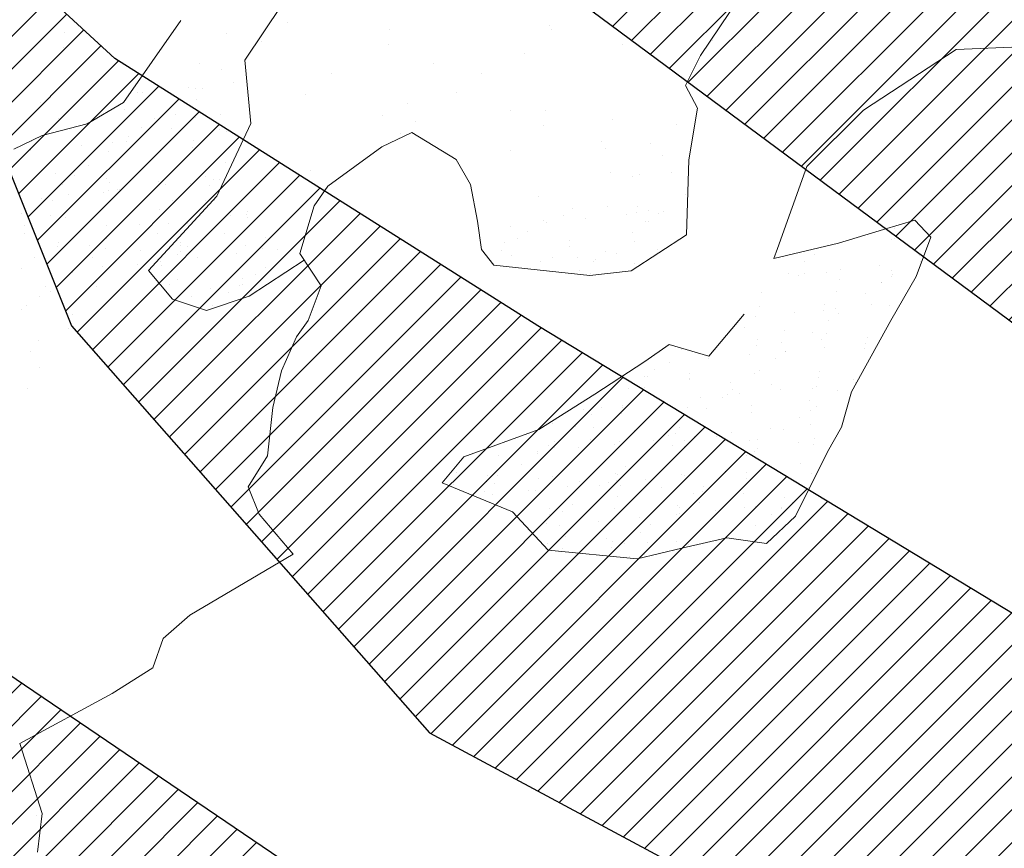
# Model space of a CAD drawing. Units: inches. Extents: x 1986 to 21484, y -1816 to 2016.
# Tile 63 of 85: x 3655.81 to 3662.33, y 1889.501 to 1894.988. Entities that reach past the tile are written whole.
import ezdxf

# ---------------------------------------------------------------- set-up
doc = ezdxf.new("R2010")
doc.units = ezdxf.units.IN
doc.layers.add('L-PLNT', color=84, linetype='Continuous', lineweight=13)
doc.layers.add('vfolhas', color=114, linetype='Continuous', lineweight=5)
doc.layers.add('vfolha2', color=110, linetype='Continuous')
doc.layers.add('vfolhas2', color=102, linetype='Continuous')
pattern_1 = [(45, (-2446.5133113, 50.986076), (-0.004419417382, 0.004419417382), [])]

# ---------------------------------------------------------------- blocks, each defined once
blk = doc.blocks.new('arbusto_PB_verde_grande')
at = {"layer": 'vfolha2'}
h = blk.add_hatch(dxfattribs=at)
h.set_pattern_fill('ANSI31', color=256, scale=0.05, style=0)
h.set_pattern_definition(pattern_1)
h.paths.add_polyline_path([(0.02944, 0.35651), (0.00028, 0.09048), (0.02625, -0.03934), (0.047, 0.06233), (0.06189, 0.09731), (0.09372, 0.26573), (0.09955, 0.43473), (0.08789, 0.61313), (0.0645, 0.72266), (0.04988, 0.6851), (0.0236, 0.51294)])
h.paths.add_polyline_path([(0.30106, 0.43789), (0.14225, 0.24871), (0.26685, 0.30022)])
h.paths.add_polyline_path([(0.37995, 0.22817), (0.23697, 0.15193), (0.18428, 0.09364), (0.11122, 0.04358), (0.02625, -0.03934), (0.28061, 0.04667), (0.36829, 0.07798), (0.46756, 0.11239), (0.61068, 0.19376), (0.71585, 0.27823), (0.55813, 0.25948)])
h.paths.add_polyline_path([(0.56101, -0.29441), (0.72752, -0.32573), (0.59024, -0.2412), (0.42962, -0.15982), (0.02625, -0.03934), (0.14922, -0.14107), (0.18838, -0.16604), (0.41501, -0.24435)])
h.paths.add_polyline_path([(-0.27429, -0.44776), (-0.30352, -0.72628), (-0.23923, -0.64175), (-0.15457, -0.45716), (0.02625, -0.03934), (-0.16328, -0.25376)])
h.paths.add_polyline_path([(-0.51963, -0.24744), (-0.67736, -0.32573), (-0.59558, -0.35072), (-0.40574, -0.32882), (-0.21007, -0.20995), (0.02625, -0.03934), (-0.14874, -0.06595), (-0.31518, -0.09101), (-0.41452, -0.15048)])
h.paths.add_polyline_path([(-0.52546, 0.25007), (-0.70947, 0.24698), (-0.51963, 0.1093), (-0.32979, 0.02167), (-0.07567, -0.0128), (-0.04234, -0.02148), (-0.35024, 0.1312)])
h = blk.add_hatch(dxfattribs=at)
h.set_pattern_fill('ANSI31', color=256, scale=0.05, style=0)
h.set_pattern_definition(pattern_1)
h.paths.add_polyline_path([(-0.18963, 0.29704), (-0.08553, 0.20192), (-0.10785, 0.25007), (-0.13202, 0.31865), (-0.25096, 0.48479), (-0.44952, 0.5505), (-0.37946, 0.43789)])
h.paths.add_polyline_path([(0.07911, -0.4071), (0.08214, -0.50631), (0.17255, -0.6355), (0.18428, -0.44151), (0.14904, -0.29177), (0.02625, -0.03934), (0.03527, -0.25376)])
at = {"layer": 'vfolhas'}
h = blk.add_hatch(dxfattribs=at)
h.set_pattern_fill('ANSI31', color=256, scale=0.05, style=0)
h.set_pattern_definition(pattern_1)
h.paths.add_polyline_path([(-0.07279, 0.50669), (-0.18085, 0.65063), (-0.2334, 0.67253), (-0.20712, 0.53176), (-0.10785, 0.25007), (0.02625, -0.03934), (0.00028, 0.09048), (0.00816, 0.16241), (-0.04939, 0.29079)])
h.paths.add_polyline_path([(0.09902, 0.41929), (0.09372, 0.26573), (0.07906, 0.18814), (0.15506, 0.36901), (0.26606, 0.5505), (0.28356, 0.63504), (0.2485, 0.68819), (0.25145, 0.63504), (0.20178, 0.54426)])
h.paths.add_polyline_path([(0.12295, 0.24073), (0.047, 0.06233), (0.02625, -0.03934), (0.11122, 0.04358), (0.18428, 0.09364), (0.27478, 0.19376), (0.3215, 0.25323), (0.44129, 0.38467), (0.47634, 0.57866), (0.41789, 0.45347), (0.28939, 0.30954)])
h.paths.add_polyline_path([(0.58145, -0.03779), (0.70707, 0.01536), (0.78591, 0.04667), (0.74796, 0.06549), (0.62818, 0.08423), (0.52595, 0.09048), (0.39745, 0.04358), (0.02625, -0.03934), (0.25728, -0.03154), (0.43834, -0.0347)])
h.paths.add_polyline_path([(0.52022, -0.03647), (0.43834, -0.0347), (0.25728, -0.03154), (0.02625, -0.03934), (0.17964, -0.08515), (0.53768, -0.13167), (0.69541, -0.15357), (0.78591, -0.07852), (0.70413, -0.10042)])
h.paths.add_polyline_path([(0.27189, -0.21929), (0.14922, -0.14107), (0.02625, -0.03934), (0.15794, -0.31007), (0.29522, -0.42585), (0.41789, -0.49157), (0.56396, -0.56669), (0.5114, -0.48532), (0.39456, -0.34139)])
h.paths.add_polyline_path([(-0.05818, -0.47591), (-0.02312, -0.61984), (0.047, -0.80134), (0.08494, -0.59794), (0.07911, -0.4071), (0.03527, -0.25376), (0.02625, -0.03934), (-0.03773, -0.26001)])
h.paths.add_polyline_path([(-0.24218, 0.14054), (-0.11073, 0.06858), (0.02625, -0.03934), (-0.04235, 0.10871), (-0.21007, 0.23757), (-0.36485, 0.33145), (-0.47874, 0.40341), (-0.54303, 0.46288), (-0.49041, 0.33145), (-0.39408, 0.22192)])
at = {"layer": 'vfolha2'}
for p, q in [((-0.37946, 0.43789), (-0.18963, 0.29704)), ((-0.52546, 0.25007), (-0.35024, 0.1312))]:
    blk.add_line(p, q, dxfattribs=at)
at = {"layer": 'vfolhas2'}
for p, q in [((-0.54303, 0.46288), (-0.49041, 0.33145)), ((-0.47874, 0.40341), (-0.54303, 0.46288)), ((-0.36485, 0.33145), (-0.47874, 0.40341)), ((-0.49041, 0.33145), (-0.39408, 0.22192)), ((-0.21007, 0.23757), (-0.36485, 0.33145)), ((-0.39408, 0.22192), (-0.24218, 0.14054))]:
    blk.add_line(p, q, dxfattribs=at)
blk = doc.blocks.new('PLANT-SHRUB')
for p, q in [((2164.0917, 1878.6487), (2164.5363, 1878.8153)), ((2164.5363, 1878.8153), (2164.8003, 1878.8153)), ((2164.8003, 1878.8153), (2164.967, 1878.607)), ((2164.8003, 1878.8153), (2164.8003, 1878.8153)), ((2164.3454, 1878.7354), (2164.3454, 1878.7354)), ((2164.4894, 1878.7345), (2164.4894, 1878.7345)), ((2164.2631, 1878.6802), (2164.2631, 1878.6802)), ((2164.5043, 1878.672), (2164.5043, 1878.672)), ((2164.5625, 1878.7068), (2164.5625, 1878.7068)), ((2164.5717, 1878.7149), (2164.5717, 1878.7149)), ((2164.6457, 1878.6958), (2164.6457, 1878.6958)), ((2164.7757, 1878.6787), (2164.7757, 1878.6787)), ((2164.9028, 1878.6857), (2164.9028, 1878.6857)), ((2163.9111, 1878.5931), (2164.0917, 1878.6487)), ((2164.967, 1878.607), (2165.231, 1878.4543)), ((2163.7026, 1878.4682), (2163.9111, 1878.5931)), ((2164.124, 1878.5527), (2164.124, 1878.5527)), ((2164.2732, 1878.5846), (2164.2732, 1878.5846)), ((2164.6821, 1878.5866), (2164.6821, 1878.5866)), ((2164.7437, 1878.5398), (2164.7437, 1878.5398)), ((2163.1885, 1878.3016), (2163.7026, 1878.4682)), ((2163.7026, 1878.4682), (2163.7026, 1878.4682)), ((2164.0946, 1878.5257), (2164.0946, 1878.5257)), ((2164.1874, 1878.4701), (2164.1874, 1878.4701)), ((2164.6853, 1878.4692), (2164.6853, 1878.4692)), ((2165.1831, 1878.4683), (2165.1831, 1878.4683)), ((2163.6377, 1878.4146), (2163.6377, 1878.4146)), ((2163.6385, 1878.4401), (2163.6385, 1878.4401)), ((2164.0475, 1878.4421), (2164.0475, 1878.4421)), ((2164.4793, 1878.4265), (2164.4793, 1878.4265)), ((2164.6046, 1878.4124), (2164.6046, 1878.4124)), ((2164.8978, 1878.4212), (2164.8978, 1878.4212)), ((2165.2243, 1878.3995), (2165.2243, 1878.3995)), ((2165.231, 1878.4543), (2165.495, 1878.3016)), ((2163.7676, 1878.3975), (2163.7676, 1878.3975)), ((2163.9355, 1878.3799), (2163.9355, 1878.3799)), ((2163.9848, 1878.3689), (2163.9848, 1878.3689)), ((2164.068, 1878.358), (2164.068, 1878.358)), ((2164.198, 1878.3409), (2164.198, 1878.3409)), ((2164.5752, 1878.3854), (2164.5752, 1878.3854)), ((2162.869, 1878.2044), (2163.1885, 1878.3016)), ((2163.1885, 1878.3016), (2163.1885, 1878.3016)), ((2163.3794, 1878.2735), (2163.3794, 1878.2735)), ((2163.4129, 1878.2975), (2163.4129, 1878.2975)), ((2163.4468, 1878.3164), (2163.4468, 1878.3164)), ((2163.8446, 1878.2819), (2163.8446, 1878.2819)), ((2163.8773, 1878.2725), (2163.8773, 1878.2725)), ((2163.9447, 1878.3155), (2163.9447, 1878.3155)), ((2164.2631, 1878.2766), (2164.2631, 1878.2766)), ((2164.3751, 1878.2716), (2164.3751, 1878.2716)), ((2164.4151, 1878.3123), (2164.4151, 1878.3123)), ((2164.4426, 1878.3146), (2164.4426, 1878.3146)), ((2164.4983, 1878.3013), (2164.4983, 1878.3013)), ((2164.6283, 1878.2842), (2164.6283, 1878.2842)), ((2164.6721, 1878.2786), (2164.6721, 1878.2786)), ((2164.873, 1878.2707), (2164.873, 1878.2707)), ((2164.9404, 1878.3137), (2164.9404, 1878.3137)), ((2165.0852, 1878.2721), (2165.0852, 1878.2721)), ((2165.3708, 1878.2698), (2165.3708, 1878.2698)), ((2165.4383, 1878.3128), (2165.4383, 1878.3128)), ((2165.495, 1878.3016), (2165.8841, 1877.8573)), ((2162.6189, 1878.0794), (2162.869, 1878.2044)), ((2163.1272, 1878.22), (2163.1272, 1878.22)), ((2163.1272, 1878.22), (2163.1272, 1878.22)), ((2163.7669, 1878.2255), (2163.7669, 1878.2255)), ((2163.7964, 1878.2525), (2163.7964, 1878.2525)), ((2164.416, 1878.2396), (2164.416, 1878.2396)), ((2164.8455, 1878.2556), (2164.8455, 1878.2556)), ((2164.9287, 1878.2447), (2164.9287, 1878.2447)), ((2165.0558, 1878.2451), (2165.0558, 1878.2451)), ((2165.0586, 1878.2275), (2165.0586, 1878.2275)), ((2165.1039, 1878.263), (2165.1039, 1878.263)), ((2165.5223, 1878.2577), (2165.5223, 1878.2577)), ((2162.7782, 1878.153), (2162.7782, 1878.153)), ((2165.2758, 1878.199), (2165.2758, 1878.199)), ((2165.359, 1878.188), (2165.359, 1878.188)), ((2165.489, 1878.1709), (2165.489, 1878.1709)), ((2162.6189, 1877.9267), (2162.6189, 1878.0794)), ((2162.7596, 1878.1163), (2162.7596, 1878.1163)), ((2162.9767, 1878.0877), (2162.9767, 1878.0877)), ((2162.9767, 1878.0877), (2162.9767, 1878.0877)), ((2162.9881, 1878.0925), (2162.9881, 1878.0925)), ((2162.9881, 1878.0925), (2162.9881, 1878.0925)), ((2163.0599, 1878.0768), (2163.0599, 1878.0768)), ((2163.0599, 1878.0768), (2163.0599, 1878.0768)), ((2163.21, 1878.1374), (2163.21, 1878.1374)), ((2163.6078, 1878.0796), (2163.6078, 1878.0796)), ((2163.6285, 1878.1321), (2163.6285, 1878.1321)), ((2164.0374, 1878.134), (2164.0374, 1878.134)), ((2164.2475, 1878.0851), (2164.2475, 1878.0851)), ((2164.277, 1878.1121), (2164.277, 1878.1121)), ((2164.4692, 1878.1185), (2164.4692, 1878.1185)), ((2164.8877, 1878.1131), (2164.8877, 1878.1131)), ((2164.8966, 1878.0993), (2164.8966, 1878.0993)), ((2165.2966, 1878.1151), (2165.2966, 1878.1151)), ((2165.5363, 1878.1048), (2165.5363, 1878.1048)), ((2165.5658, 1878.1318), (2165.5658, 1878.1318)), ((2162.9587, 1878.0655), (2162.9587, 1878.0655)), ((2162.9587, 1878.0655), (2162.9587, 1878.0655)), ((2163.0626, 1878.0716), (2163.0626, 1878.0716)), ((2163.0626, 1878.0716), (2163.0626, 1878.0716)), ((2163.1899, 1878.0596), (2163.1899, 1878.0596)), ((2163.4071, 1878.0311), (2163.4071, 1878.0311)), ((2163.4903, 1878.0201), (2163.4903, 1878.0201)), ((2163.5604, 1878.0707), (2163.5604, 1878.0707)), ((2164.0583, 1878.0698), (2164.0583, 1878.0698)), ((2164.5561, 1878.0689), (2164.5561, 1878.0689)), ((2165.054, 1878.068), (2165.054, 1878.068)), ((2165.5518, 1878.0671), (2165.5518, 1878.0671)), ((2162.9938, 1877.9875), (2162.9938, 1877.9875)), ((2162.9938, 1877.9875), (2162.9938, 1877.9875)), ((2163.4028, 1877.9895), (2163.4028, 1877.9895)), ((2163.4687, 1877.9522), (2163.4687, 1877.9522)), ((2163.6202, 1878.003), (2163.6202, 1878.003)), ((2163.8346, 1877.9739), (2163.8346, 1877.9739)), ((2163.8374, 1877.9744), (2163.8374, 1877.9744)), ((2163.9206, 1877.9634), (2163.9206, 1877.9634)), ((2164.0506, 1877.9463), (2164.0506, 1877.9463)), ((2164.253, 1877.9686), (2164.253, 1877.9686)), ((2164.662, 1877.9705), (2164.662, 1877.9705)), ((2164.7281, 1877.9448), (2164.7281, 1877.9448)), ((2164.7575, 1877.9718), (2164.7575, 1877.9718)), ((2165.0938, 1877.955), (2165.0938, 1877.955)), ((2165.3772, 1877.959), (2165.3772, 1877.959)), ((2165.5123, 1877.9496), (2165.5123, 1877.9496)), ((2162.8134, 1877.8295), (2162.6189, 1877.9267)), ((2162.7995, 1877.9197), (2162.7995, 1877.9197)), ((2162.7995, 1877.9197), (2162.7995, 1877.9197)), ((2162.8199, 1877.917), (2162.8199, 1877.917)), ((2162.8199, 1877.917), (2162.8199, 1877.917)), ((2163.3177, 1877.9161), (2163.3177, 1877.9161)), ((2163.4392, 1877.9252), (2163.4392, 1877.9252)), ((2163.8156, 1877.9152), (2163.8156, 1877.9152)), ((2164.0884, 1877.9393), (2164.0884, 1877.9393)), ((2164.2677, 1877.9177), (2164.2677, 1877.9177)), ((2164.3134, 1877.9143), (2164.3134, 1877.9143)), ((2164.3509, 1877.9068), (2164.3509, 1877.9068)), ((2164.4809, 1877.8897), (2164.4809, 1877.8897)), ((2164.8113, 1877.9134), (2164.8113, 1877.9134)), ((2165.3091, 1877.9125), (2165.3091, 1877.9125)), ((2165.807, 1877.9116), (2165.807, 1877.9116)), ((2162.7525, 1877.874), (2162.7525, 1877.874)), ((2162.7525, 1877.874), (2162.7525, 1877.874)), ((2163.0913, 1877.6907), (2162.8134, 1877.8295)), ((2163.1999, 1877.8294), (2163.1999, 1877.8294)), ((2163.2503, 1877.8731), (2163.2503, 1877.8731)), ((2163.6184, 1877.824), (2163.6184, 1877.824)), ((2163.7482, 1877.8722), (2163.7482, 1877.8722)), ((2164.0274, 1877.826), (2164.0274, 1877.826)), ((2164.246, 1877.8713), (2164.246, 1877.8713)), ((2164.6981, 1877.8611), (2164.6981, 1877.8611)), ((2164.7439, 1877.8704), (2164.7439, 1877.8704)), ((2164.7813, 1877.8501), (2164.7813, 1877.8501)), ((2164.9112, 1877.833), (2164.9112, 1877.833)), ((2165.2381, 1877.8315), (2165.2381, 1877.8315)), ((2165.2417, 1877.8695), (2165.2417, 1877.8695)), ((2165.7396, 1877.8686), (2165.7396, 1877.8686)), ((2165.8578, 1877.8187), (2165.8578, 1877.8187)), ((2165.8841, 1877.8573), (2165.8841, 1877.5102)), ((2163.2801, 1877.7794), (2163.2801, 1877.7794)), ((2163.9198, 1877.7849), (2163.9198, 1877.7849)), ((2163.9493, 1877.8119), (2163.9493, 1877.8119)), ((2164.4591, 1877.8104), (2164.4591, 1877.8104)), ((2164.569, 1877.799), (2164.569, 1877.799)), ((2164.8776, 1877.8051), (2164.8776, 1877.8051)), ((2165.1284, 1877.8044), (2165.1284, 1877.8044)), ((2165.2087, 1877.8045), (2165.2087, 1877.8045)), ((2165.2116, 1877.7935), (2165.2116, 1877.7935)), ((2165.2866, 1877.807), (2165.2866, 1877.807)), ((2165.3416, 1877.7764), (2165.3416, 1877.7764)), ((2165.5587, 1877.7478), (2165.5587, 1877.7478)), ((2165.7184, 1877.7915), (2165.7184, 1877.7915)), ((2163.4729, 1877.4726), (2163.0913, 1877.6907)), ((2165.6419, 1877.7368), (2165.6419, 1877.7368)), ((2165.7187, 1877.6912), (2165.7187, 1877.6912)), ((2165.7719, 1877.7197), (2165.7719, 1877.7197)), ((2163.2597, 1877.6365), (2163.2597, 1877.6365)), ((2163.3429, 1877.6256), (2163.3429, 1877.6256)), ((2163.3927, 1877.6814), (2163.3927, 1877.6814)), ((2163.4313, 1877.6704), (2163.4313, 1877.6704)), ((2163.7607, 1877.6391), (2163.7607, 1877.6391)), ((2163.8245, 1877.6659), (2163.8245, 1877.6659)), ((2164.2306, 1877.649), (2163.8694, 1877.6074)), ((2163.9292, 1877.6695), (2163.9292, 1877.6695)), ((2164.3696, 1877.413), (2164.2306, 1877.649)), ((2164.243, 1877.6605), (2164.243, 1877.6605)), ((2164.4004, 1877.6446), (2164.4004, 1877.6446)), ((2164.427, 1877.6686), (2164.427, 1877.6686)), ((2164.4299, 1877.6716), (2164.4299, 1877.6716)), ((2164.6519, 1877.6625), (2164.6519, 1877.6625)), ((2164.9249, 1877.6676), (2164.9249, 1877.6676)), ((2165.0495, 1877.6587), (2165.0495, 1877.6587)), ((2165.0837, 1877.6469), (2165.0837, 1877.6469)), ((2165.4227, 1877.6667), (2165.4227, 1877.6667)), ((2165.5022, 1877.6416), (2165.5022, 1877.6416)), ((2165.6892, 1877.6642), (2165.6892, 1877.6642)), ((2161.3267, 1877.5657), (2161.6462, 1877.2881)), ((2163.4729, 1877.6085), (2163.4729, 1877.6085)), ((2163.69, 1877.5799), (2163.69, 1877.5799)), ((2164.3335, 1877.4952), (2164.3335, 1877.4952)), ((2164.4491, 1877.5024), (2164.4491, 1877.5024)), ((2164.6822, 1877.513), (2164.6822, 1877.513)), ((2164.8675, 1877.497), (2164.8675, 1877.497)), ((2164.881, 1877.5043), (2164.881, 1877.5043)), ((2164.9105, 1877.5313), (2164.9105, 1877.5313)), ((2165.18, 1877.5121), (2165.18, 1877.5121)), ((2165.2765, 1877.499), (2165.2765, 1877.499)), ((2165.5301, 1877.5184), (2165.5301, 1877.5184)), ((2165.6779, 1877.5112), (2165.6779, 1877.5112)), ((2165.8841, 1877.5102), (2166.0925, 1877.052)), ((2162.8967, 1877.177), (2163.4108, 1877.4408)), ((2163.4108, 1877.4408), (2163.4729, 1877.4726)), ((2163.4108, 1877.4408), (2163.4108, 1877.4408)), ((2164.5507, 1877.4666), (2164.5507, 1877.4666)), ((2164.6148, 1877.4701), (2164.6148, 1877.4701)), ((2164.6339, 1877.4556), (2164.6339, 1877.4556)), ((2164.7638, 1877.4385), (2164.7638, 1877.4385)), ((2165.1126, 1877.4692), (2165.1126, 1877.4692)), ((2165.6105, 1877.4683), (2165.6105, 1877.4683)), ((2165.7083, 1877.4835), (2165.7083, 1877.4835)), ((2164.5641, 1877.3852), (2164.3696, 1877.413)), ((2164.5641, 1877.3852), (2164.5641, 1877.3852)), ((2164.9531, 1877.3158), (2164.5641, 1877.3852)), ((2164.7219, 1877.3585), (2164.7219, 1877.3585)), ((2164.981, 1877.4099), (2164.981, 1877.4099)), ((2165.0642, 1877.399), (2165.0642, 1877.399)), ((2165.1942, 1877.3819), (2165.1942, 1877.3819)), ((2165.3616, 1877.3639), (2165.3616, 1877.3639)), ((2165.391, 1877.391), (2165.391, 1877.391)), ((2165.3839, 1877.2325), (2164.9531, 1877.3158)), ((2165.0736, 1877.3389), (2165.0736, 1877.3389)), ((2165.4113, 1877.3533), (2165.4113, 1877.3533)), ((2165.4921, 1877.3336), (2165.4921, 1877.3336)), ((2165.4945, 1877.3423), (2165.4945, 1877.3423)), ((2165.6245, 1877.3252), (2165.6245, 1877.3252)), ((2165.8416, 1877.2966), (2165.8416, 1877.2966)), ((2165.9011, 1877.3355), (2165.9011, 1877.3355)), ((2161.6462, 1877.2881), (2162.3688, 1877.1631)), ((2165.2936, 1877.2664), (2165.2936, 1877.2664)), ((2165.8702, 1877.0243), (2165.3839, 1877.2325)), ((2165.7915, 1877.2655), (2165.7915, 1877.2655)), ((2165.8716, 1877.2506), (2165.8716, 1877.2506)), ((2165.9249, 1877.2857), (2165.9249, 1877.2857)), ((2162.3688, 1877.1631), (2162.8967, 1877.177)), ((2165.6982, 1877.1754), (2165.6982, 1877.1754)), ((2165.8422, 1877.2236), (2165.8422, 1877.2236)), ((2166.0466, 1877.11), (2166.0466, 1877.11)), ((2166.0925, 1877.052), (2165.8702, 1877.0243)), ((2165.9792, 1877.067), (2165.9792, 1877.067)), ((2165.891, 1877.0275), (2165.891, 1877.0275)), ((2169.5216, 1876.8362), (2169.7195, 1877.001)), ((2163.4361, 1876.6098), (2163.7885, 1876.9619)), ((2163.7885, 1876.9619), (2164.2179, 1876.8849)), ((2163.9971, 1876.9019), (2163.9971, 1876.9019)), ((2164.1688, 1876.8679), (2164.1688, 1876.8679)), ((2164.2179, 1876.8849), (2164.4382, 1876.7198)), ((2169.3127, 1876.3968), (2169.5216, 1876.8362)), ((2169.5557, 1876.8206), (2169.5557, 1876.8206)), ((2163.6084, 1876.7628), (2163.6084, 1876.7628)), ((2163.7943, 1876.7418), (2163.7943, 1876.7418)), ((2163.8255, 1876.7342), (2163.8255, 1876.7342)), ((2163.9087, 1876.7232), (2163.9087, 1876.7232)), ((2163.9261, 1876.7133), (2163.9261, 1876.7133)), ((2164.0387, 1876.7061), (2164.0387, 1876.7061)), ((2164.0665, 1876.7579), (2164.0665, 1876.7579)), ((2164.2128, 1876.7364), (2164.2128, 1876.7364)), ((2164.424, 1876.7124), (2164.424, 1876.7124)), ((2164.4382, 1876.7198), (2164.8566, 1876.2357)), ((2164.4382, 1876.7198), (2164.4382, 1876.7198)), ((2167.1158, 1876.3736), (2167.1332, 1876.7213)), ((2167.1332, 1876.7213), (2167.9098, 1876.5474)), ((2163.8587, 1876.6703), (2163.8587, 1876.6703)), ((2164.2559, 1876.6775), (2164.2559, 1876.6775)), ((2164.3391, 1876.6666), (2164.3391, 1876.6666)), ((2164.3565, 1876.6694), (2164.3565, 1876.6694)), ((2164.469, 1876.6495), (2164.469, 1876.6495)), ((2163.1608, 1876.4008), (2163.4361, 1876.6098)), ((2163.5781, 1876.5919), (2163.5781, 1876.5919)), ((2163.898, 1876.6035), (2163.898, 1876.6035)), ((2163.9274, 1876.6305), (2163.9274, 1876.6305)), ((2163.9871, 1876.5938), (2163.9871, 1876.5938)), ((2164.4189, 1876.5783), (2164.4189, 1876.5783)), ((2168.1447, 1876.5387), (2168.3274, 1876.6343)), ((2168.3274, 1876.6343), (2168.6406, 1876.5735)), ((2167.9098, 1876.5474), (2168.1447, 1876.5387)), ((2168.6406, 1876.5735), (2169.3127, 1876.3968)), ((2163.5418, 1876.4685), (2163.5418, 1876.4685)), ((2163.7389, 1876.4577), (2163.7389, 1876.4577)), ((2164.0397, 1876.4676), (2164.0397, 1876.4676)), ((2164.3786, 1876.4632), (2164.3786, 1876.4632)), ((2164.408, 1876.4902), (2164.408, 1876.4902)), ((2164.5375, 1876.4667), (2164.5375, 1876.4667)), ((2163.1168, 1876.2357), (2163.1608, 1876.4008)), ((2163.3381, 1876.3844), (2163.3381, 1876.3844)), ((2163.7842, 1876.4337), (2163.7842, 1876.4337)), ((2164.2027, 1876.4284), (2164.2027, 1876.4284)), ((2164.6116, 1876.4303), (2164.6116, 1876.4303)), ((2169.3127, 1876.3968), (2169.3127, 1876.3968)), ((2163.5462, 1876.357), (2163.5462, 1876.357)), ((2163.8711, 1876.3143), (2163.8711, 1876.3143)), ((2164.2194, 1876.3174), (2164.2194, 1876.3174)), ((2167.0462, 1876.191), (2167.1158, 1876.3736)), ((2164.2948, 1876.3121), (2164.2948, 1876.3121)), ((2164.4088, 1876.2702), (2164.4088, 1876.2702)), ((2164.7253, 1876.2682), (2164.7253, 1876.2682)), ((2164.8273, 1876.2649), (2164.8273, 1876.2649)), ((2162.9076, 1876.1587), (2163.1168, 1876.2357)), ((2164.414, 1876.2428), (2164.414, 1876.2428)), ((2164.5388, 1876.2264), (2164.5388, 1876.2264)), ((2164.622, 1876.2154), (2164.622, 1876.2154)), ((2164.752, 1876.1983), (2164.752, 1876.1983)), ((2164.8566, 1876.2357), (2164.8456, 1876.1037)), ((2166.8113, 1876.1302), (2167.0462, 1876.191)), ((2162.4231, 1876.0487), (2162.9076, 1876.1587)), ((2162.7811, 1876.1406), (2162.7811, 1876.1406)), ((2163.7742, 1876.1257), (2163.7742, 1876.1257)), ((2163.7875, 1876.1768), (2163.7875, 1876.1768)), ((2164.6016, 1876.1223), (2164.6016, 1876.1223)), ((2164.7, 1876.1771), (2164.7, 1876.1771)), ((2166.5677, 1875.9215), (2166.8113, 1876.1302)), ((2162.7074, 1876.0731), (2162.7074, 1876.0731)), ((2163.619, 1876.0694), (2163.619, 1876.0694)), ((2164.3302, 1876.1085), (2164.3302, 1876.1085)), ((2164.8456, 1876.1037), (2164.7355, 1875.9497)), ((2164.7355, 1875.9497), (2164.6033, 1875.7406)), ((2166.3589, 1875.7824), (2166.5677, 1875.9215)), ((2163.2337, 1875.751), (2163.2337, 1875.751)), ((2163.9825, 1875.7899), (2163.9825, 1875.7899)), ((2164.2561, 1875.7559), (2164.2561, 1875.7559)), ((2164.6033, 1875.7406), (2164.5593, 1875.5536)), ((2166.1327, 1875.6868), (2166.3589, 1875.7824)), ((2163.9088, 1875.7224), (2163.9088, 1875.7224)), ((2166.0022, 1875.6607), (2166.1327, 1875.6868)), ((2165.7839, 1875.5525), (2166.0022, 1875.6607)), ((2164.0715, 1875.5625), (2164.0715, 1875.5625)), ((2164.5593, 1875.5536), (2164.6497, 1875.2224)), ((2165.7398, 1875.2994), (2165.7839, 1875.5525)), ((2163.511, 1875.3578), (2163.511, 1875.3578)), ((2163.749, 1875.3556), (2163.749, 1875.3556)), ((2166.1777, 1875.2758), (2165.7487, 1875.3505)), ((2163.5026, 1875.328), (2163.5026, 1875.328)), ((2165.4535, 1875.1344), (2165.7398, 1875.2994)), ((2165.7398, 1875.2994), (2165.7398, 1875.2994)), ((2166.4493, 1875.1525), (2166.1777, 1875.2758)), ((2164.0455, 1875.2565), (2164.0455, 1875.2565)), ((2164.2535, 1875.2291), (2164.2535, 1875.2291)), ((2164.6497, 1875.2224), (2164.8589, 1875.1564)), ((2165.9653, 1875.2107), (2165.9653, 1875.2107)), ((2166.1416, 1875.2621), (2166.1416, 1875.2621)), ((2164.5784, 1875.1863), (2164.5784, 1875.1863)), ((2164.7094, 1875.1737), (2164.7094, 1875.1737)), ((2164.8589, 1875.1564), (2165.2994, 1875.1014)), ((2164.8589, 1875.1564), (2164.8589, 1875.1564)), ((2165.8306, 1875.1793), (2165.8306, 1875.1793)), ((2166.0485, 1875.1998), (2166.0485, 1875.1998)), ((2166.1261, 1875.1611), (2166.1261, 1875.1611)), ((2166.1556, 1875.1881), (2166.1556, 1875.1881)), ((2166.1785, 1875.1826), (2166.1785, 1875.1826)), ((2166.2624, 1875.1637), (2166.2624, 1875.1637)), ((2166.3956, 1875.1541), (2166.3956, 1875.1541)), ((2166.5603, 1874.9428), (2166.4493, 1875.1525)), ((2165.2994, 1875.1014), (2165.4535, 1875.1344)), ((2165.8989, 1875.1075), (2165.8989, 1875.1075)), ((2166.3968, 1875.1066), (2166.3968, 1875.1066)), ((2164.5408, 1875.0663), (2164.5408, 1875.0663)), ((2165.8315, 1875.0645), (2165.8315, 1875.0645)), ((2165.967, 1875.0153), (2165.967, 1875.0153)), ((2166.0462, 1875.0138), (2166.0462, 1875.0138)), ((2166.3293, 1875.0636), (2166.3293, 1875.0636)), ((2166.4552, 1875.0158), (2166.4552, 1875.0158)), ((2164.2309, 1874.9858), (2164.2309, 1874.9858)), ((2164.7125, 1875.0071), (2164.7125, 1875.0071)), ((2165.3104, 1874.9469), (2165.3104, 1874.9469)), ((2165.8279, 1874.8879), (2165.8279, 1874.8879)), ((2166.548, 1874.6962), (2166.5603, 1874.9428)), ((2165.7985, 1874.8609), (2165.7985, 1874.8609)), ((2165.8205, 1874.8712), (2165.8205, 1874.8712)), ((2166.0125, 1874.8617), (2166.0125, 1874.8617)), ((2166.2523, 1874.8557), (2166.2523, 1874.8557)), ((2166.4476, 1874.875), (2166.4476, 1874.875)), ((2166.5103, 1874.8608), (2166.5103, 1874.8608)), ((2165.9011, 1874.8052), (2165.9011, 1874.8052)), ((2166.0311, 1874.7881), (2166.0311, 1874.7881)), ((2166.2482, 1874.7595), (2166.2482, 1874.7595)), ((2166.3315, 1874.7486), (2166.3315, 1874.7486)), ((2164.3648, 1874.6884), (2164.3648, 1874.6884)), ((2165.8816, 1874.6469), (2166.548, 1874.6962)), ((2166.2676, 1874.7062), (2166.2676, 1874.7062)), ((2166.2791, 1874.7205), (2166.2791, 1874.7205)), ((2166.3085, 1874.7475), (2166.3085, 1874.7475)), ((2166.4451, 1874.7077), (2166.4451, 1874.7077)), ((2166.4614, 1874.7315), (2166.4614, 1874.7315)), ((2167.6651, 1874.7188), (2167.6651, 1874.7188)), ((2164.2911, 1874.6209), (2164.2911, 1874.6209)), ((2165.3879, 1874.4496), (2165.8816, 1874.6469)), ((2165.914, 1874.6563), (2165.914, 1874.6563)), ((2166.148, 1874.6455), (2166.148, 1874.6455)), ((2167.5132, 1874.67), (2167.5132, 1874.67)), ((2164.77, 1874.5721), (2164.77, 1874.5721)), ((2164.9933, 1874.5594), (2164.9933, 1874.5594)), ((2165.7924, 1874.577), (2165.7924, 1874.577)), ((2165.8209, 1874.5551), (2165.8209, 1874.5551)), ((2165.8699, 1874.5636), (2165.8699, 1874.5636)), ((2165.9541, 1874.6173), (2165.9541, 1874.6173)), ((2166.238, 1874.5571), (2166.238, 1874.5571)), ((2166.3321, 1874.5576), (2166.3321, 1874.5576)), ((2166.4922, 1874.5625), (2166.4922, 1874.5625)), ((2166.5765, 1874.6162), (2166.5765, 1874.6162)), ((2167.1145, 1874.5614), (2167.1145, 1874.5614)), ((2167.1988, 1874.6151), (2167.1988, 1874.6151)), ((2167.4826, 1874.5549), (2167.4826, 1874.5549)), ((2165.683, 1874.5235), (2165.683, 1874.5235)), ((2165.8455, 1874.5021), (2165.8455, 1874.5021)), ((2166.7855, 1874.5038), (2166.7855, 1874.5038)), ((2166.8718, 1874.5382), (2166.8718, 1874.5382)), ((2166.8718, 1874.5382), (2166.8718, 1874.5382)), ((2167.3949, 1874.5315), (2167.3949, 1874.5315)), ((2165.1287, 1874.1166), (2165.3879, 1874.4496)), ((2165.9491, 1874.4632), (2165.9491, 1874.4632)), ((2166.1169, 1874.4664), (2166.1169, 1874.4664)), ((2166.2209, 1874.4527), (2166.2209, 1874.4527)), ((2166.3834, 1874.4313), (2166.3834, 1874.4313)), ((2166.7487, 1874.4701), (2166.7487, 1874.4701)), ((2165.5388, 1874.3769), (2165.5388, 1874.3769)), ((2166.0785, 1874.3575), (2166.0785, 1874.3575)), ((2166.6548, 1874.3956), (2166.6548, 1874.3956)), ((2166.7588, 1874.3819), (2166.7588, 1874.3819)), ((2166.9213, 1874.3605), (2166.9213, 1874.3605)), ((2165.5663, 1874.3377), (2165.5663, 1874.3377)), ((2165.7752, 1874.3039), (2165.7752, 1874.3039)), ((2166.0961, 1874.3102), (2166.0961, 1874.3102)), ((2166.6016, 1874.3508), (2166.6016, 1874.3508)), ((2166.7184, 1874.3091), (2166.7184, 1874.3091)), ((2167.1128, 1874.3532), (2167.1128, 1874.3532)), ((2167.1154, 1874.3055), (2167.1154, 1874.3055)), ((2167.1927, 1874.3248), (2167.1927, 1874.3248)), ((2167.2967, 1874.3111), (2167.2967, 1874.3111)), ((2167.3407, 1874.3079), (2167.3407, 1874.3079)), ((2165.4926, 1874.2702), (2165.4926, 1874.2702)), ((2165.7384, 1874.2702), (2165.7384, 1874.2702)), ((2166.5498, 1874.2878), (2166.5498, 1874.2878)), ((2165.2852, 1874.1768), (2165.2852, 1874.1768)), ((2165.6312, 1874.1706), (2165.6312, 1874.1706)), ((2165.8083, 1874.1701), (2165.8083, 1874.1701)), ((2166.3195, 1874.1726), (2166.3195, 1874.1726)), ((2166.3314, 1874.1634), (2166.3314, 1874.1634)), ((2166.8758, 1874.1683), (2166.8758, 1874.1683)), ((2164.6968, 1874.018), (2165.1287, 1874.1166)), ((2164.7528, 1874.1286), (2164.7528, 1874.1286)), ((2164.9608, 1874.1012), (2164.9608, 1874.1012)), ((2165.7927, 1874.1169), (2165.7927, 1874.1169)), ((2166.376, 1874.1285), (2166.376, 1874.1285)), ((2166.4151, 1874.1158), (2166.4151, 1874.1158)), ((2166.8592, 1874.1531), (2166.8592, 1874.1531)), ((2167.0374, 1874.1147), (2167.0374, 1874.1147)), ((2167.1505, 1874.1124), (2167.1505, 1874.1124)), ((2165.2858, 1874.0584), (2165.2858, 1874.0584)), ((2165.4627, 1874.0632), (2165.4627, 1874.0632)), ((2165.5395, 1874.0879), (2165.5395, 1874.0879)), ((2165.7085, 1874.0632), (2165.7085, 1874.0632)), ((2166.3308, 1874.0621), (2166.3308, 1874.0621)), ((2166.3391, 1874.0948), (2166.3391, 1874.0948)), ((2166.7073, 1874.061), (2166.7073, 1874.061)), ((2166.9531, 1874.061), (2166.9531, 1874.061)), ((2165.4987, 1874.0304), (2165.4987, 1874.0304)), ((2165.5262, 1873.9919), (2165.5262, 1873.9919)), ((2165.6612, 1874.009), (2165.6612, 1874.009)), ((2165.8286, 1873.9869), (2165.8286, 1873.9869)), ((2165.9326, 1873.9732), (2165.9326, 1873.9732)), ((2166.0659, 1873.9724), (2166.0659, 1873.9724)), ((2166.7677, 1873.9869), (2166.7677, 1873.9869)), ((2165.0948, 1873.9056), (2165.0948, 1873.9056)), ((2165.3656, 1873.9286), (2165.3656, 1873.9286)), ((2166.0367, 1873.9596), (2166.0367, 1873.9596)), ((2166.0367, 1873.9596), (2166.0367, 1873.9596)), ((2166.1402, 1873.9125), (2166.1402, 1873.9125)), ((2166.1991, 1873.9382), (2166.1991, 1873.9382)), ((2166.3616, 1873.9168), (2166.3616, 1873.9168)), ((2166.4706, 1873.9024), (2166.4706, 1873.9024)), ((2166.589, 1873.9657), (2166.589, 1873.9657)), ((2166.6941, 1873.9194), (2166.6941, 1873.9194)), ((2166.9399, 1873.9194), (2166.9399, 1873.9194)), ((2166.9767, 1873.9531), (2166.9767, 1873.9531)), ((2166.5746, 1873.8887), (2166.5746, 1873.8887)), ((2166.737, 1873.8673), (2166.737, 1873.8673)), ((2166.9045, 1873.8453), (2166.9045, 1873.8453)), ((2165.2583, 1873.6357), (2165.9062, 1873.7713)), ((2165.7672, 1873.807), (2165.7672, 1873.807)), ((2165.7957, 1873.7851), (2165.7957, 1873.7851)), ((2165.9062, 1873.7713), (2166.1777, 1873.7097)), ((2165.9347, 1873.8098), (2165.9347, 1873.8098)), ((2166.3069, 1873.7875), (2166.3069, 1873.7875)), ((2166.557, 1873.8087), (2166.557, 1873.8087)), ((2166.1777, 1873.7097), (2166.4493, 1873.5617)), ((2166.1777, 1873.7097), (2166.1777, 1873.7097)), ((2166.741, 1873.7371), (2166.741, 1873.7371)), ((2166.5671, 1873.5778), (2166.5671, 1873.5778)), ((2166.5764, 1873.5807), (2166.5764, 1873.5807)), ((2165.9152, 1873.5563), (2165.9152, 1873.5563)), ((2166.2963, 1873.5549), (2166.2963, 1873.5549)), ((2166.4493, 1873.5617), (2166.6467, 1873.5)), ((2166.5303, 1873.5441), (2166.5303, 1873.5441)), ((2166.3062, 1873.3933), (2166.3062, 1873.3933)), ((2165.9485, 1873.2362), (2165.9485, 1873.2362)), ((2165.8749, 1873.1687), (2165.8749, 1873.1687))]:
    blk.add_line(p, q)

msp = doc.modelspace()

# ---------------------------------------------------------------- block references
at = {"layer": 'L-PLNT', "rotation": 223.1883365522388}
msp.add_blockref('PLANT-SHRUB', (3953.27, 4742.9646), dxfattribs=at)
at = {"layer": 'L-PLNT', "xscale": 24.60366729364114, "yscale": 24.60366729364114, "zscale": 24.60366729364114}
msp.add_blockref('arbusto_PB_verde_grande', (3668.2184, 1884.8051), dxfattribs=at)

doc.saveas('drawing.dxf')
